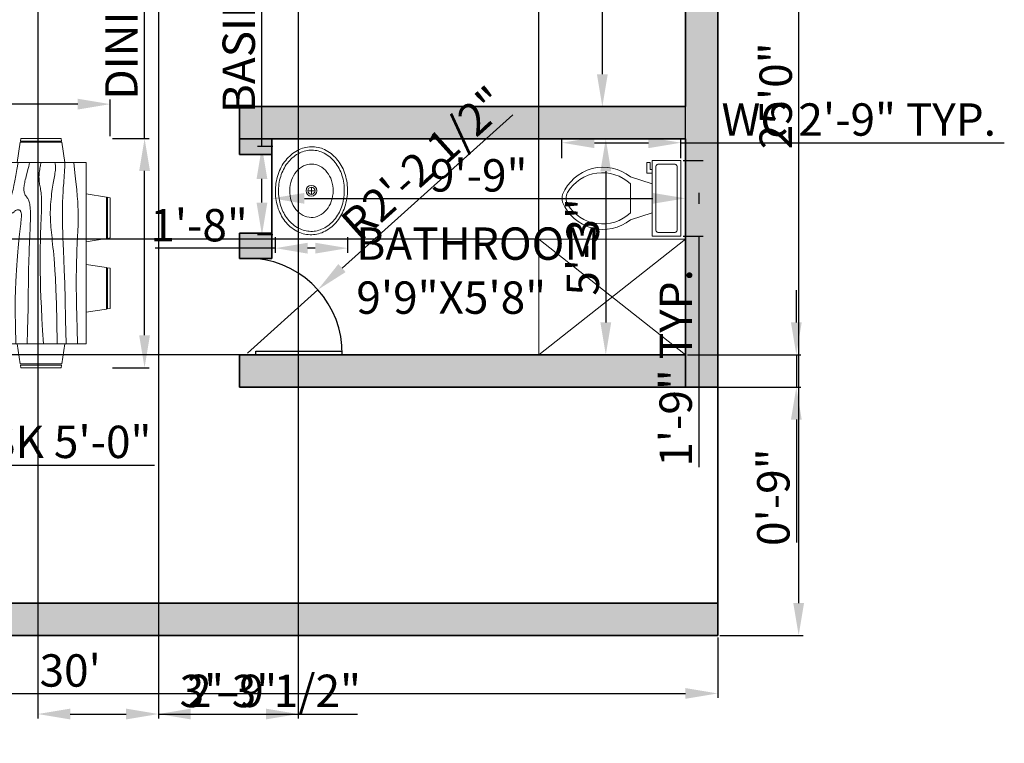
# Model space of a CAD drawing. Units: inches. Extents: x 39700 to 40173, y 40700 to 41139.
# Tile 3 of 4: x 39899 to 40173, y 40718 to 40919. Entities that reach past the tile are written whole.
import ezdxf

# ---------------------------------------------------------------- set-up
doc = ezdxf.new("R2010")
doc.units = ezdxf.units.IN
for name, color, linetype, lineweight in [('A-ANNO-DIMS', 2, 'Continuous', 18), ('A-AREA-IDEN', 7, 'Continuous', 25), ('A-DOOR', 4, 'Continuous', 25), ('A-FLOR-FIXT', 9, 'Continuous', 18), ('A-FURN', 8, 'Continuous', 18), ('A-WALL', 7, 'Continuous', 35)]:
    doc.layers.add(name, color=color, linetype=linetype, lineweight=lineweight)
doc.layers.add('A-WALL-PATT', color=251, linetype='Continuous', lineweight=13, true_color=0x636466)
doc.styles.get("Standard").update_dxf_attribs({"font": 'arial.ttf'})
doc.dimstyles.new('ISO-25', dxfattribs={"dimtxt": 9, "dimasz": 9, "dimexe": 1.25, "dimexo": 0.625, "dimtad": 1, "dimdec": 1, "dimrnd": 9, "dimlunit": 3, "dimtxsty": 'Standard', "dimcen": 2.5, "dimadec": 0, "dimazin": 0, "dimtfac": 1, "dimtdec": 1, "dimtmove": 0, "dimatfit": 3, "dimfxl": 1, "dimarcsym": 0})

# ---------------------------------------------------------------- blocks, each defined once
blk = doc.blocks.new('*D6')
at = {"layer": 'A-ANNO-DIMS', "color": 0, "lineweight": -2, "transparency": 16777216}
for p, q in [((40083.8, 41039.04), (40060.09, 41039.04)), ((40061.34, 41030.04), (40061.34, 40904.04)), ((40083.8, 40895.04), (40060.09, 40895.04))]:
    blk.add_line(p, q, dxfattribs=at)
at = {"layer": 'A-ANNO-DIMS', "color": 0, "transparency": 16777216}
for points in [[(40059.84, 41030.04), (40062.84, 41030.04), (40061.34, 41039.04)], [(40059.84, 40904.04), (40062.84, 40904.04), (40061.34, 40895.04)]]:
    blk.add_solid(points, dxfattribs=at)
at = {"layer": 'Defpoints', "color": 0, "transparency": 16777216}
for p in [(40084.42, 41039.04), (40061.34, 40895.04), (40084.42, 40895.04)]:
    blk.add_point(p, dxfattribs=at)
at = {"layer": 'A-ANNO-DIMS', "color": 0, "transparency": 16777216, "insert": (40056.19, 40967.04), "char_height": 9, "attachment_point": 5, "rotation": 90}
blk.add_mtext("12'", dxfattribs=at)
blk = doc.blocks.new('*D7')
at = {"layer": 'A-ANNO-DIMS', "color": 0, "lineweight": -2, "transparency": 16777216}
for p, q in [((40083.8, 40886.04), (40061.05, 40886.04)), ((40062.3, 40877.04), (40062.3, 40835.04)), ((40083.8, 40826.04), (40061.05, 40826.04))]:
    blk.add_line(p, q, dxfattribs=at)
at = {"layer": 'A-ANNO-DIMS', "color": 0, "transparency": 16777216}
for points in [[(40060.8, 40877.04), (40063.8, 40877.04), (40062.3, 40886.04)], [(40060.8, 40835.04), (40063.8, 40835.04), (40062.3, 40826.04)]]:
    blk.add_solid(points, dxfattribs=at)
at = {"layer": 'Defpoints', "color": 0, "transparency": 16777216}
for p in [(40084.42, 40886.04), (40062.3, 40826.04), (40084.42, 40826.04)]:
    blk.add_point(p, dxfattribs=at)
at = {"layer": 'A-ANNO-DIMS', "color": 0, "transparency": 16777216, "insert": (40057.08, 40856.04), "char_height": 9, "attachment_point": 5, "rotation": 90}
blk.add_mtext('5\'-3"', dxfattribs=at)
blk = doc.blocks.new('*D10')
at = {"layer": 'A-ANNO-DIMS', "color": 0, "lineweight": -2, "transparency": 16777216}
for p, q in [((40094.05, 41048.04), (40117.17, 41048.04)), ((40115.92, 40757.04), (40115.92, 41039.04)), ((40094.05, 40748.04), (40117.17, 40748.04))]:
    blk.add_line(p, q, dxfattribs=at)
at = {"layer": 'A-ANNO-DIMS', "color": 0, "transparency": 16777216}
for points in [[(40114.42, 41039.04), (40117.42, 41039.04), (40115.92, 41048.04)], [(40114.42, 40757.04), (40117.42, 40757.04), (40115.92, 40748.04)]]:
    blk.add_solid(points, dxfattribs=at)
at = {"layer": 'Defpoints', "color": 0, "transparency": 16777216}
for p in [(40093.42, 41048.04), (40115.92, 41048.04), (40093.42, 40748.04)]:
    blk.add_point(p, dxfattribs=at)
at = {"layer": 'A-ANNO-DIMS', "color": 0, "transparency": 16777216, "insert": (40110.7, 40898.04), "char_height": 9, "attachment_point": 5, "rotation": 90}
blk.add_mtext('25\'0"', dxfattribs=at)
blk = doc.blocks.new('Toilet - top')
for p, q in [((9.5, -6), (9.5, -2)), ((-8, -8.5), (-8, -8)), ((-7, -8), (-7, -9.5)), ((-4, -8), (-6, -14)), ((4, -8), (6, -14)), ((-10, -8.5), (-8, -8.5)), ((-10, -9.5), (-10, -8.5)), ((-7, -9.5), (-10, -9.5)), ((4, -14), (-4, -14))]:
    blk.add_line(p, q)
blk.add_lwpolyline([(10.5, -8), (10.5, 0), (-10.5, 0), (-10.5, -8)], close=True)
for points in [[(-9.5, -2), (-9.5, -6)], [(8.5, -1), (-8.5, -1)], [(-8.5, -7), (8.5, -7)]]:
    blk.add_lwpolyline(points)
for centre, radius, start, end in [((-8.62, -1.88), 0.884, 81.8699, 188.1301), ((8.62, -1.88), 0.884, 351.8699, 98.1301), ((-8.62, -6.12), 0.884, 171.8699, 278.1301), ((8.62, -6.12), 0.884, 261.8699, 8.1301), ((3.52, -21.58), 12.17, 141.4691, 247.9714), ((4.2, -21.82), 11.33, 136.3677, 238.9468), ((-3.52, -21.58), 12.17, 292.0284, 38.5307), ((-4.2, -21.82), 11.33, 301.053, 43.6321), ((0, -27.88), 4, 245.7318, 294.2682), ((0, -29), 4, 254.8605, 285.1395)]:
    blk.add_arc(centre, radius, start, end)
blk = doc.blocks.new('*D20')
at = {"layer": 'A-ANNO-DIMS', "color": 0, "lineweight": -2, "transparency": 16777216}
for p, q in [((39969.51, 40881.12), (39969.51, 40868.28)), ((40084.42, 40881.12), (40084.42, 40868.28)), ((39978.51, 40869.53), (40075.42, 40869.53))]:
    blk.add_line(p, q, dxfattribs=at)
at = {"layer": 'A-ANNO-DIMS', "color": 0, "transparency": 16777216}
for points in [[(39978.51, 40871.03), (39978.51, 40868.03), (39969.51, 40869.53)], [(40075.42, 40871.03), (40075.42, 40868.03), (40084.42, 40869.53)]]:
    blk.add_solid(points, dxfattribs=at)
at = {"layer": 'Defpoints', "color": 0, "transparency": 16777216}
for p in [(39969.51, 40881.75), (40084.42, 40881.75), (40084.42, 40869.53)]:
    blk.add_point(p, dxfattribs=at)
at = {"layer": 'A-ANNO-DIMS', "color": 0, "transparency": 16777216, "insert": (40026.97, 40874.75), "char_height": 9, "attachment_point": 5}
blk.add_mtext('9\'-9"', dxfattribs=at)
blk = doc.blocks.new('Dining Set - 36 x 72 in.')
for p, q in [((-22, 27.5), (-22.1562, 26.50042)), ((-22, 27.5), (-6, 27.5)), ((-5.8437, 26.49966), (-6, 27.5)), ((6, 27.5), (5.8438, 26.50042)), ((6, 27.5), (22, 27.5)), ((22.1563, 26.49966), (22, 27.5)), ((-22.2343, 26.00059), (-23.4847, 17.99762)), ((-22.2304, 26), (-5.7608, 26)), ((-5.8416, 26.5), (-22.1534, 26.5)), ((-4.5152, 17.99762), (-5.7655, 25.99926)), ((5.7657, 26.00059), (4.5153, 17.99762)), ((5.7696, 26), (22.2392, 26)), ((22.1584, 26.5), (5.8466, 26.5)), ((23.4848, 17.99762), (22.2345, 25.99926)), ((36, 18), (-36, 18)), ((-36, 18), (-36, -18)), ((36, -18), (36, 18)), ((-45.5, 8), (-44.5004, 8.15617)), ((-45.5, 8), (-45.5, -8)), ((-44.5, -8.15843), (-44.5, 8.15338)), ((-44.0006, 8.23428), (-35.9976, 9.48474)), ((-44, 8.23041), (-44, -8.23915)), ((44.0006, 8.23428), (35.9976, 9.48474)), ((44, 8.23041), (44, -8.23915)), ((44.5, -8.15843), (44.5, 8.15338)), ((45.5, 8), (44.5005, 8.15617)), ((45.5, 8), (45.5, -8)), ((-44.4997, -8.15631), (-45.5, -8)), ((-35.9976, -9.48476), (-43.9993, -8.2345)), ((35.9976, -9.48476), (43.9993, -8.2345)), ((44.4997, -8.15631), (45.5, -8)), ((-36, -18), (36, -18)), ((-22.2343, -26.0006), (-23.4847, -17.99762)), ((-4.5152, -17.99762), (-5.7655, -25.99928)), ((5.7657, -26.0006), (4.5153, -17.99762)), ((23.4848, -17.99762), (22.2345, -25.99928)), ((-22.2304, -26), (-5.7608, -26)), ((-22, -27.5), (-22.1562, -26.50044)), ((-5.8416, -26.5), (-22.1534, -26.5)), ((-5.8437, -26.49967), (-6, -27.5)), ((5.7696, -26), (22.2392, -26)), ((6, -27.5), (5.8438, -26.50044)), ((22.1584, -26.5), (5.8466, -26.5)), ((22.1563, -26.49967), (22, -27.5)), ((-22, -27.5), (-6, -27.5)), ((6, -27.5), (22, -27.5))]:
    blk.add_line(p, q)
for points in [[(-36, 15), (-31.1772, 14.97754), (-26.8079, 14.91406), (-22.8538, 14.81543), (-19.276, 14.6875), (-16.0362, 14.53613), (-13.0957, 14.36718), (-10.4159, 14.18652), (-7.9583, 14), (-5.6904, 13.81315), (-3.6035, 13.63021), (-1.6954, 13.45508), (0.0365, 13.29166), (1.5945, 13.14388), (2.9811, 13.01562), (4.1988, 12.9108), (5.25, 12.83333), (6.1393, 12.78613), (6.8802, 12.76823), (7.4883, 12.77767), (7.9792, 12.8125), (8.3685, 12.87077), (8.6719, 12.95052), (8.9049, 13.0498), (9.0833, 13.16666), (9.2205, 13.29899), (9.3216, 13.44401), (9.3895, 13.59879), (9.4271, 13.76041), (9.4373, 13.92594), (9.4232, 14.09245), (9.3875, 14.257), (9.3333, 14.41666), (9.2638, 14.56917), (9.1836, 14.71484), (9.0975, 14.85465), (9.0104, 14.98958), (8.9272, 15.1206), (8.8529, 15.2487), (8.7922, 15.37483), (8.75, 15.5), (8.7305, 15.62467), (8.7344, 15.74739), (8.7617, 15.86621), (8.8125, 15.97916), (8.8867, 16.08431), (8.9844, 16.17968), (9.1055, 16.26334), (9.25, 16.33333), (9.4189, 16.38802), (9.6172, 16.42708), (9.8506, 16.45052), (10.125, 16.45833), (10.4463, 16.45052), (10.8203, 16.42708), (11.2529, 16.38802), (11.75, 16.33333), (12.3184, 16.26318), (12.9694, 16.17838), (13.7151, 16.07991), (14.5677, 15.96875), (15.5395, 15.84586), (16.6426, 15.71224), (17.8893, 15.56884), (19.2917, 15.41666), (20.859, 15.25667), (22.5879, 15.08984), (24.4721, 14.91715), (26.5052, 14.73958), (28.6809, 14.5581), (30.9929, 14.3737), (33.4347, 14.18733), (36, 14)], [(-36, 10), (-28.9766, 10.14274), (-23.1725, 10.20442), (-18.4241, 10.19775), (-14.5677, 10.13541), (-11.4399, 10.03011), (-8.877, 9.89453), (-6.7154, 9.74137), (-4.7917, 9.58333), (-2.9698, 9.43082), (-1.2246, 9.28515), (0.4415, 9.14534), (2.026, 9.01041), (3.5266, 8.87939), (4.9408, 8.7513), (6.266, 8.62516), (7.5, 8.5), (8.6411, 8.37549), (9.6914, 8.2539), (10.6538, 8.13818), (11.5312, 8.03125), (12.3267, 7.93603), (13.043, 7.85547), (13.6831, 7.79248), (14.25, 7.75), (14.7471, 7.7303), (15.1797, 7.73307), (15.5537, 7.75732), (15.875, 7.80208), (16.1494, 7.86637), (16.3828, 7.94922), (16.5811, 8.04964), (16.75, 8.16666), (16.8944, 8.29915), (17.0143, 8.44531), (17.1089, 8.60319), (17.1771, 8.77083), (17.218, 8.94629), (17.2305, 9.1276), (17.2137, 9.31282), (17.1667, 9.5), (17.0895, 9.6875), (16.987, 9.875), (16.8649, 10.0625), (16.7292, 10.25), (16.5856, 10.4375), (16.4401, 10.625), (16.2985, 10.8125), (16.1667, 11), (16.05, 11.18733), (15.9518, 11.3737), (15.8752, 11.5581), (15.8229, 11.73958), (15.798, 11.91715), (15.8034, 12.08984), (15.842, 12.25667), (15.9167, 12.41666), (16.0295, 12.56836), (16.1784, 12.70833), (16.3605, 12.83268), (16.5729, 12.9375), (16.8127, 13.01888), (17.0768, 13.07291), (17.3625, 13.0957), (17.6667, 13.08333), (17.9894, 13.03312), (18.3418, 12.94726), (18.7382, 12.82918), (19.1927, 12.68229), (19.7195, 12.51001), (20.3327, 12.31575), (21.0465, 12.10294), (21.875, 11.875), (22.8357, 11.63354), (23.959, 11.37304), (25.2786, 11.08618), (26.8282, 10.76562), (28.6414, 10.40405), (30.752, 9.99414), (33.1936, 9.52856), (36, 9)], [(-36, 5.5), (-30.7157, 5.3348), (-26.069, 5.20963), (-21.9946, 5.11767), (-18.4271, 5.05208), (-15.3009, 5.00602), (-12.5508, 4.97265), (-10.1112, 4.94515), (-7.9167, 4.91666), (-5.909, 4.88167), (-4.0586, 4.83984), (-2.3429, 4.79215), (-0.7396, 4.73958), (0.7739, 4.6831), (2.22, 4.6237), (3.6213, 4.56233), (5, 4.5), (6.373, 4.43782), (7.7344, 4.3776), (9.0723, 4.32129), (10.375, 4.27083), (11.6309, 4.22819), (12.8281, 4.19531), (13.9551, 4.17415), (15, 4.16666), (15.954, 4.17448), (16.819, 4.19791), (17.6001, 4.23698), (18.3021, 4.29166), (18.9299, 4.36198), (19.4883, 4.44791), (19.9823, 4.54948), (20.4167, 4.66666), (20.7969, 4.79899), (21.1302, 4.94401), (21.4245, 5.09879), (21.6875, 5.26041), (21.9271, 5.42594), (22.1511, 5.59245), (22.3672, 5.757), (22.5834, 5.91666), (22.8065, 6.06868), (23.0404, 6.21093), (23.2879, 6.34147), (23.5521, 6.45833), (23.8358, 6.55957), (24.142, 6.64323), (24.4735, 6.70735), (24.8334, 6.75), (25.2235, 6.76969), (25.642, 6.76692), (26.0858, 6.74267), (26.5521, 6.69791), (27.0379, 6.63362), (27.5404, 6.55078), (28.0565, 6.45036), (28.5834, 6.33333), (29.1242, 6.19987), (29.7071, 6.04687), (30.3661, 5.87044), (31.1354, 5.66666), (32.0493, 5.43164), (33.142, 5.16146), (34.4475, 4.85221), (36, 4.5)], [(-36, -1), (-30.7915, -0.6591), (-26.0195, -0.38216), (-21.6519, -0.16284), (-17.6563, 0.00521), (-14.0005, 0.12833), (-10.6523, 0.21289), (-7.5796, 0.26522), (-4.75, 0.29166), (-2.134, 0.29793), (0.2878, 0.28711), (2.5317, 0.26163), (4.6146, 0.22396), (6.5529, 0.17651), (8.3633, 0.12174), (10.0623, 0.06209), (11.6667, 0), (13.1899, -0.06201), (14.6341, -0.1211), (15.9982, -0.17432), (17.2813, -0.21875), (18.4823, -0.25147), (19.6003, -0.26953), (20.6343, -0.27002), (21.5834, -0.25), (22.4481, -0.20768), (23.2357, -0.14584), (23.9549, -0.06836), (24.6146, 0.02083), (25.2235, 0.11784), (25.7904, 0.21875), (26.3241, 0.31966), (26.8334, 0.41666), (27.3265, 0.50618), (27.8099, 0.58593), (28.2894, 0.65397), (28.7709, 0.70833), (29.2601, 0.74707), (29.763, 0.76823), (30.2855, 0.76985), (30.8334, 0.75), (31.4088, 0.70784), (31.9994, 0.64713), (32.589, 0.57275), (33.1615, 0.48958), (33.7008, 0.4025), (34.1908, 0.3164), (34.6153, 0.23616), (34.9584, 0.16666), (35.2099, 0.11165), (35.3848, 0.07031), (35.504, 0.04069), (35.5886, 0.02083), (35.6594, 0.00879), (35.7377, 0.0026), (35.8442, 0.00032), (36, 0)], [(-36, -6.5), (-27.1843, -6.31267), (-20.084, -6.1263), (-14.469, -5.9419), (-10.1094, -5.76042), (-6.7752, -5.58285), (-4.2363, -5.41016), (-2.2629, -5.24333), (-0.625, -5.08334), (0.8708, -4.93099), (2.2715, -4.78646), (3.5872, -4.64974), (4.8281, -4.52084), (6.0046, -4.39974), (7.127, -4.28646), (8.2053, -4.18099), (9.25, -4.08334), (10.2705, -3.99382), (11.2734, -3.91407), (12.2647, -3.84603), (13.25, -3.79167), (14.2354, -3.75293), (15.2266, -3.73177), (16.2295, -3.73015), (17.25, -3.75), (18.2912, -3.79248), (19.3451, -3.85547), (20.4009, -3.93604), (21.4479, -4.03125), (22.4754, -4.13819), (23.4727, -4.25391), (24.4289, -4.37549), (25.3334, -4.5), (26.1785, -4.62492), (26.9694, -4.74935), (27.7145, -4.87281), (28.4219, -4.99479), (29.1, -5.11483), (29.7572, -5.23242), (30.4016, -5.34709), (31.0417, -5.45834), (31.6837, -5.56437), (32.3262, -5.65821), (32.9658, -5.73153), (33.599, -5.77604), (34.2224, -5.78345), (34.8327, -5.74545), (35.4264, -5.65373), (36, -5.5)], [(-36, -10), (-26.4022, -9.81299), (-18.4675, -9.62891), (-11.9839, -9.45069), (-6.7396, -9.28125), (-2.5226, -9.12354), (0.8789, -8.98047), (3.6769, -8.85498), (6.0833, -8.75), (8.2767, -8.66765), (10.3021, -8.60677), (12.1712, -8.56543), (13.8958, -8.54167), (15.4876, -8.53353), (16.9583, -8.53907), (18.3197, -8.55632), (19.5834, -8.58334), (20.7616, -8.61841), (21.8685, -8.66081), (22.9188, -8.71004), (23.9271, -8.76563), (24.9081, -8.82707), (25.8763, -8.89388), (26.8465, -8.96558), (27.8334, -9.04167), (28.8474, -9.12118), (29.8828, -9.20117), (30.93, -9.27824), (31.9792, -9.34896), (33.0205, -9.40991), (34.0443, -9.45768), (35.0407, -9.48885), (36, -9.5)], [(-36, -14.5), (-30.0881, -14.33513), (-25.0332, -14.21224), (-20.7312, -14.12647), (-17.0781, -14.07292), (-13.97, -14.04671), (-11.3027, -14.04297), (-8.9724, -14.05681), (-6.875, -14.08334), (-4.9224, -14.11833), (-3.0905, -14.16016), (-1.3709, -14.20785), (0.2448, -14.26042), (1.7647, -14.3169), (3.1973, -14.3763), (4.5507, -14.43767), (5.8333, -14.5), (7.0554, -14.5621), (8.235, -14.62175), (9.3922, -14.67652), (10.5469, -14.72396), (11.7192, -14.76164), (12.929, -14.78711), (14.1965, -14.79794), (15.5417, -14.79167), (16.9933, -14.76424), (18.6152, -14.70508), (20.4804, -14.60197), (22.6615, -14.44271), (25.2312, -14.21509), (28.2624, -13.9069), (31.8277, -13.50594), (36, -13)]]:
    blk.add_lwpolyline(points)
blk = doc.blocks.new('*D21')
at = {"layer": 'A-ANNO-DIMS', "color": 0, "lineweight": -2, "transparency": 16777216}
for p, q in [((39733.42, 40747.42), (39733.42, 40730.66)), ((40093.42, 40747.42), (40093.42, 40730.66)), ((39742.42, 40731.91), (40084.42, 40731.91))]:
    blk.add_line(p, q, dxfattribs=at)
at = {"layer": 'A-ANNO-DIMS', "color": 0, "transparency": 16777216}
for points in [[(39742.42, 40733.41), (39742.42, 40730.41), (39733.42, 40731.91)], [(40084.42, 40733.41), (40084.42, 40730.41), (40093.42, 40731.91)]]:
    blk.add_solid(points, dxfattribs=at)
at = {"layer": 'Defpoints', "color": 0, "transparency": 16777216}
for p in [(39733.42, 40748.04), (40093.42, 40748.04), (40093.42, 40731.91)]:
    blk.add_point(p, dxfattribs=at)
at = {"layer": 'A-ANNO-DIMS', "color": 0, "transparency": 16777216, "insert": (39913.42, 40737.13), "char_height": 9, "attachment_point": 5}
blk.add_mtext("30'", dxfattribs=at)
blk = doc.blocks.new('Sink - Oval top')
for p, q in [((-1, 0), (1, 0)), ((0, 1), (0, -1))]:
    blk.add_line(p, q)
for points in [[(-12.23, 0.39, 0.117634), (-11.46, -3.36, 0.104469), (-8.88, -6.8, 0.090016), (-5.08, -9.07, 0.08192), (-0.32, -10.02, 0.08192), (4.49, -9.38, 0.090016), (8.42, -7.36, 0.104469), (11.22, -4.09, 0.117634), (12.23, -0.39, 0.117634), (11.46, 3.36, 0.104469), (8.88, 6.8, 0.090016), (5.08, 9.07, 0.08192), (0.32, 10.02, 0.08192), (-4.49, 9.38, 0.090016), (-8.42, 7.36, 0.104469), (-11.22, 4.09, 0.117634)], [(-11.29, 0.16, 0.118622), (-10.52, -3.25, 0.104678), (-8.07, -6.36, 0.089562), (-4.54, -8.37, 0.081185), (-0.13, -9.15, 0.081185), (4.3, -8.49, 0.089562), (7.89, -6.58, 0.104678), (10.42, -3.55, 0.118622), (11.29, -0.16, 0.118622), (10.52, 3.25, 0.104678), (8.07, 6.36, 0.089562), (4.54, 8.37, 0.081185), (0.13, 9.15, 0.081185), (-4.3, 8.49, 0.089562), (-7.89, 6.58, 0.104678), (-10.42, 3.55, 0.118622)], [(-7.42, 0.08, 0.118283), (-6.91, -2.17, 0.104607), (-5.29, -4.21, 0.089718), (-2.97, -5.53, 0.081436), (-0.07, -6.04, 0.081436), (2.84, -5.59, 0.089718), (5.2, -4.33, 0.104607), (6.86, -2.32, 0.118283), (7.42, -0.08, 0.118283), (6.91, 2.17, 0.104607), (5.29, 4.21, 0.089718), (2.97, 5.53, 0.081436), (0.07, 6.04, 0.081436), (-2.84, 5.59, 0.089718), (-5.2, 4.33, 0.104607), (-6.86, 2.32, 0.118283)]]:
    blk.add_lwpolyline(points, format="xyb", close=True)
for radius in [1.5, 1]:
    blk.add_circle((0, 0), radius)
blk = doc.blocks.new('*D22')
at = {"layer": 'A-ANNO-DIMS', "color": 0, "lineweight": -2, "transparency": 16777216}
for p, q in [((40050.12, 40880.66), (40050.12, 40886.24)), ((40059.12, 40884.99), (40074.17, 40884.99)), ((40083.17, 40880.66), (40083.17, 40886.24)), ((40083.17, 40884.99), (40173.08, 40884.99))]:
    blk.add_line(p, q, dxfattribs=at)
at = {"layer": 'A-ANNO-DIMS', "color": 0, "transparency": 16777216}
for points in [[(40059.12, 40886.49), (40059.12, 40883.49), (40050.12, 40884.99)], [(40074.17, 40886.49), (40074.17, 40883.49), (40083.17, 40884.99)]]:
    blk.add_solid(points, dxfattribs=at)
at = {"layer": 'Defpoints', "color": 0, "transparency": 16777216}
for p in [(40083.17, 40884.99), (40050.12, 40880.03), (40083.17, 40880.03)]:
    blk.add_point(p, dxfattribs=at)
at = {"layer": 'A-ANNO-DIMS', "color": 0, "transparency": 16777216, "insert": (40132.62, 40890.27), "char_height": 9, "attachment_point": 5}
blk.add_mtext('WC 2\'-9" TYP.', dxfattribs=at)
blk = doc.blocks.new('*D23')
at = {"layer": 'A-ANNO-DIMS', "color": 0, "lineweight": -2, "transparency": 16777216}
for p, q in [((40083.79, 40880.03), (40089.37, 40880.03)), ((40088.12, 40871.03), (40088.12, 40868.03)), ((40083.79, 40859.03), (40089.37, 40859.03)), ((40088.12, 40859.03), (40088.12, 40794.77))]:
    blk.add_line(p, q, dxfattribs=at)
at = {"layer": 'A-ANNO-DIMS', "color": 0, "transparency": 16777216}
for points in [[(40086.62, 40871.03), (40089.62, 40871.03), (40088.12, 40880.03)], [(40086.62, 40868.03), (40089.62, 40868.03), (40088.12, 40859.03)]]:
    blk.add_solid(points, dxfattribs=at)
at = {"layer": 'Defpoints', "color": 0, "transparency": 16777216}
for p in [(40083.17, 40880.03), (40083.17, 40859.03), (40088.12, 40859.03)]:
    blk.add_point(p, dxfattribs=at)
at = {"layer": 'A-ANNO-DIMS', "color": 0, "transparency": 16777216, "insert": (40082.9, 40822.4), "char_height": 9, "attachment_point": 5, "rotation": 90}
blk.add_mtext('1\'-9" TYP.', dxfattribs=at)
blk = doc.blocks.new('*D30')
at = {"layer": 'A-ANNO-DIMS', "color": 0, "lineweight": -2, "transparency": 16777216}
for p, q in [((39934.09, 40886.16), (39934.09, 41016.31)), ((39925.16, 40886.16), (39935.34, 40886.16)), ((39934.09, 40831.46), (39934.09, 40877.16)), ((39925.16, 40822.46), (39935.34, 40822.46))]:
    blk.add_line(p, q, dxfattribs=at)
at = {"layer": 'A-ANNO-DIMS', "color": 0, "transparency": 16777216}
for points in [[(39932.59, 40877.16), (39935.59, 40877.16), (39934.09, 40886.16)], [(39932.59, 40831.46), (39935.59, 40831.46), (39934.09, 40822.46)]]:
    blk.add_solid(points, dxfattribs=at)
at = {"layer": 'Defpoints', "color": 0, "transparency": 16777216}
for p in [(39924.53, 40886.16), (39934.09, 40886.16), (39924.53, 40822.46)]:
    blk.add_point(p, dxfattribs=at)
at = {"layer": 'A-ANNO-DIMS', "color": 0, "transparency": 16777216, "insert": (39928.81, 40955.74), "char_height": 9, "attachment_point": 5, "rotation": 90}
blk.add_mtext('DINING SET 5\'-3 1/2"', dxfattribs=at)
blk = doc.blocks.new('*D31')
at = {"layer": 'A-ANNO-DIMS', "color": 0, "lineweight": -2, "transparency": 16777216}
for p, q in [((39886.03, 40895.72), (39830.89, 40895.72)), ((39886.03, 40886.79), (39886.03, 40896.97)), ((39915.53, 40895.72), (39895.03, 40895.72)), ((39924.53, 40886.79), (39924.53, 40896.97))]:
    blk.add_line(p, q, dxfattribs=at)
at = {"layer": 'A-ANNO-DIMS', "color": 0, "transparency": 16777216}
for points in [[(39895.03, 40897.22), (39895.03, 40894.22), (39886.03, 40895.72)], [(39915.53, 40897.22), (39915.53, 40894.22), (39924.53, 40895.72)]]:
    blk.add_solid(points, dxfattribs=at)
at = {"layer": 'Defpoints', "color": 0, "transparency": 16777216}
for p in [(39886.03, 40895.72), (39886.03, 40886.16), (39924.53, 40886.16)]:
    blk.add_point(p, dxfattribs=at)
at = {"layer": 'A-ANNO-DIMS', "color": 0, "transparency": 16777216, "insert": (39853.96, 40901), "char_height": 9, "attachment_point": 5}
blk.add_mtext('3\'-2 1/2"', dxfattribs=at)
blk = doc.blocks.new('*D34')
at = {"layer": 'A-ANNO-DIMS', "color": 0, "lineweight": -2, "transparency": 16777216}
for p, q in [((39805.37, 40803.76), (39805.37, 40794.14)), ((39865.37, 40803.76), (39865.37, 40794.14)), ((39814.37, 40795.39), (39856.37, 40795.39)), ((39865.37, 40795.39), (39936.83, 40795.39))]:
    blk.add_line(p, q, dxfattribs=at)
at = {"layer": 'A-ANNO-DIMS', "color": 0, "transparency": 16777216}
for points in [[(39814.37, 40796.89), (39814.37, 40793.89), (39805.37, 40795.39)], [(39856.37, 40796.89), (39856.37, 40793.89), (39865.37, 40795.39)]]:
    blk.add_solid(points, dxfattribs=at)
at = {"layer": 'Defpoints', "color": 0, "transparency": 16777216}
for p in [(39805.37, 40804.39), (39865.37, 40804.39), (39865.37, 40795.39)]:
    blk.add_point(p, dxfattribs=at)
at = {"layer": 'A-ANNO-DIMS', "color": 0, "transparency": 16777216, "insert": (39905.6, 40800.67), "char_height": 9, "attachment_point": 5}
blk.add_mtext('DESK 5\'-0"', dxfattribs=at)
blk = doc.blocks.new('*D38')
at = {"layer": 'A-ANNO-DIMS', "color": 0, "lineweight": -2, "transparency": 16777216}
for p, q in [((39966.72, 40883.91), (39966.72, 40979.88)), ((39969.78, 40883.91), (39965.47, 40883.91)), ((39966.72, 40868.36), (39966.72, 40874.91)), ((39969.78, 40859.36), (39965.47, 40859.36))]:
    blk.add_line(p, q, dxfattribs=at)
at = {"layer": 'A-ANNO-DIMS', "color": 0, "transparency": 16777216}
for points in [[(39965.22, 40874.91), (39968.22, 40874.91), (39966.72, 40883.91)], [(39965.22, 40868.36), (39968.22, 40868.36), (39966.72, 40859.36)]]:
    blk.add_solid(points, dxfattribs=at)
at = {"layer": 'Defpoints', "color": 0, "transparency": 16777216}
for p in [(39966.72, 40883.91), (39970.4, 40883.91), (39970.4, 40859.36)]:
    blk.add_point(p, dxfattribs=at)
at = {"layer": 'A-ANNO-DIMS', "color": 0, "transparency": 16777216, "insert": (39961.44, 40936.4), "char_height": 9, "attachment_point": 5, "rotation": 90}
blk.add_mtext('BASIN 2\'-0 1/2"', dxfattribs=at)
blk = doc.blocks.new('*D39')
at = {"layer": 'A-ANNO-DIMS', "color": 0, "lineweight": -2, "transparency": 16777216}
for p, q in [((39970.4, 40858.73), (39970.4, 40854.43)), ((39990.54, 40858.73), (39990.54, 40854.43)), ((39970.4, 40855.68), (39937.08, 40855.68)), ((39981.54, 40855.68), (39979.4, 40855.68))]:
    blk.add_line(p, q, dxfattribs=at)
at = {"layer": 'A-ANNO-DIMS', "color": 0, "transparency": 16777216}
for points in [[(39979.4, 40857.18), (39979.4, 40854.18), (39970.4, 40855.68)], [(39981.54, 40857.18), (39981.54, 40854.18), (39990.54, 40855.68)]]:
    blk.add_solid(points, dxfattribs=at)
at = {"layer": 'Defpoints', "color": 0, "transparency": 16777216}
for p in [(39970.4, 40859.36), (39990.54, 40859.36), (39970.4, 40855.68)]:
    blk.add_point(p, dxfattribs=at)
at = {"layer": 'A-ANNO-DIMS', "color": 0, "transparency": 16777216, "insert": (39949.24, 40860.9), "char_height": 9, "attachment_point": 5}
blk.add_mtext('1\'-8"', dxfattribs=at)
blk = doc.blocks.new('*D46')
at = {"layer": 'A-ANNO-DIMS', "color": 0, "lineweight": -2, "transparency": 16777216}
for p, q in [((40115.27, 40835.04), (40115.27, 40844.04)), ((40085.05, 40826.04), (40116.52, 40826.04)), ((40115.27, 40826.04), (40115.27, 40817.04)), ((40085.05, 40817.04), (40116.52, 40817.04)), ((40115.27, 40808.04), (40115.27, 40773.87))]:
    blk.add_line(p, q, dxfattribs=at)
at = {"layer": 'A-ANNO-DIMS', "color": 0, "transparency": 16777216}
for points in [[(40113.77, 40835.04), (40116.77, 40835.04), (40115.27, 40826.04)], [(40113.77, 40808.04), (40116.77, 40808.04), (40115.27, 40817.04)]]:
    blk.add_solid(points, dxfattribs=at)
at = {"layer": 'Defpoints', "color": 0, "transparency": 16777216}
for p in [(40084.42, 40826.04), (40084.42, 40817.04), (40115.27, 40817.04)]:
    blk.add_point(p, dxfattribs=at)
at = {"layer": 'A-ANNO-DIMS', "color": 0, "transparency": 16777216, "insert": (40110.05, 40786.46), "char_height": 9, "attachment_point": 5, "rotation": 90}
blk.add_mtext('0\'-9"', dxfattribs=at)
blk = doc.blocks.new('*D47')
at = {"layer": 'A-ANNO-DIMS', "color": 0, "lineweight": -2, "transparency": 16777216}
for p, q in [((40043.65, 40858.83), (40043.65, 41071.14)), ((40084.42, 40858.83), (40084.42, 41071.14)), ((40052.65, 41069.89), (40075.42, 41069.89))]:
    blk.add_line(p, q, dxfattribs=at)
at = {"layer": 'A-ANNO-DIMS', "color": 0, "transparency": 16777216}
for points in [[(40052.65, 41071.39), (40052.65, 41068.39), (40043.65, 41069.89)], [(40075.42, 41071.39), (40075.42, 41068.39), (40084.42, 41069.89)]]:
    blk.add_solid(points, dxfattribs=at)
at = {"layer": 'Defpoints', "color": 0, "transparency": 16777216}
for p in [(40084.42, 41069.89), (40043.65, 40858.21), (40084.42, 40858.21)]:
    blk.add_point(p, dxfattribs=at)
at = {"layer": 'A-ANNO-DIMS', "color": 0, "transparency": 16777216, "insert": (40064.03, 41075.12), "char_height": 9, "attachment_point": 5}
blk.add_mtext('3\'-5"', dxfattribs=at)
blk = doc.blocks.new('*D48')
at = {"layer": 'A-ANNO-DIMS', "color": 0, "lineweight": -2, "transparency": 16777216}
for p, q in [((40043.02, 40858.21), (39710.32, 40858.21)), ((39711.57, 40835.04), (39711.57, 40849.21)), ((40043.02, 40826.04), (39710.32, 40826.04))]:
    blk.add_line(p, q, dxfattribs=at)
at = {"layer": 'A-ANNO-DIMS', "color": 0, "transparency": 16777216}
for points in [[(39710.07, 40849.21), (39713.07, 40849.21), (39711.57, 40858.21)], [(39710.07, 40835.04), (39713.07, 40835.04), (39711.57, 40826.04)]]:
    blk.add_solid(points, dxfattribs=at)
at = {"layer": 'Defpoints', "color": 0, "transparency": 16777216}
for p in [(39711.57, 40858.21), (40043.65, 40858.21), (40043.65, 40826.04)]:
    blk.add_point(p, dxfattribs=at)
at = {"layer": 'A-ANNO-DIMS', "color": 0, "transparency": 16777216, "insert": (39706.35, 40842.12), "char_height": 9, "attachment_point": 5, "rotation": 90}
blk.add_mtext('2\'-8"', dxfattribs=at)
blk = doc.blocks.new('*D50')
at = {"layer": 'A-ANNO-DIMS', "color": 0, "lineweight": -2, "transparency": 16777216}
for p, q in [((39904.42, 40952.02), (39904.42, 40724.94)), ((39937.94, 40952.02), (39937.94, 40724.94)), ((39913.42, 40726.19), (39928.94, 40726.19)), ((39937.94, 40726.19), (39993.24, 40726.19))]:
    blk.add_line(p, q, dxfattribs=at)
at = {"layer": 'A-ANNO-DIMS', "color": 0, "transparency": 16777216}
for points in [[(39913.42, 40727.69), (39913.42, 40724.69), (39904.42, 40726.19)], [(39928.94, 40727.69), (39928.94, 40724.69), (39937.94, 40726.19)]]:
    blk.add_solid(points, dxfattribs=at)
at = {"layer": 'Defpoints', "color": 0, "transparency": 16777216}
for p in [(39904.42, 40952.64), (39937.94, 40952.64), (39937.94, 40726.19)]:
    blk.add_point(p, dxfattribs=at)
at = {"layer": 'A-ANNO-DIMS', "color": 0, "transparency": 16777216, "insert": (39970.09, 40731.47), "char_height": 9, "attachment_point": 5}
blk.add_mtext('2\'-9 1/2"', dxfattribs=at)
blk = doc.blocks.new('*D51')
at = {"layer": 'A-ANNO-DIMS', "color": 0, "lineweight": -2, "transparency": 16777216}
for p, q in [((39976.83, 40957.96), (39976.83, 40724.94)), ((39937.94, 40952.02), (39937.94, 40724.94)), ((39946.94, 40726.19), (39967.83, 40726.19))]:
    blk.add_line(p, q, dxfattribs=at)
at = {"layer": 'A-ANNO-DIMS', "color": 0, "transparency": 16777216}
for points in [[(39946.94, 40727.69), (39946.94, 40724.69), (39937.94, 40726.19)], [(39967.83, 40727.69), (39967.83, 40724.69), (39976.83, 40726.19)]]:
    blk.add_solid(points, dxfattribs=at)
at = {"layer": 'Defpoints', "color": 0, "transparency": 16777216}
for p in [(39976.83, 40958.58), (39937.94, 40952.64), (39976.83, 40726.19)]:
    blk.add_point(p, dxfattribs=at)
at = {"layer": 'A-ANNO-DIMS', "color": 0, "transparency": 16777216, "insert": (39957.39, 40731.42), "char_height": 9, "attachment_point": 5}
blk.add_mtext('3\'-3"', dxfattribs=at)
blk = doc.blocks.new('*D55')
at = {"layer": 'A-ANNO-DIMS', "color": 0, "lineweight": -2, "transparency": 16777216}
for p, q in [((40036.42, 40892.74), (39988.98, 40850.15)), ((39962.67, 40826.54), (39982.28, 40844.14))]:
    blk.add_line(p, q, dxfattribs=at)
at = {"layer": 'A-ANNO-DIMS', "color": 0, "transparency": 16777216}
blk.add_solid([(39987.97, 40851.27), (39989.98, 40849.04), (39982.28, 40844.14)], dxfattribs=at)
at = {"layer": 'Defpoints', "color": 0, "transparency": 16777216}
for p in [(39982.28, 40844.14), (39962.67, 40826.54)]:
    blk.add_point(p, dxfattribs=at)
at = {"layer": 'A-ANNO-DIMS', "color": 0, "transparency": 16777216, "insert": (40012.52, 40878.38), "char_height": 9, "attachment_point": 5, "rotation": 41.9102}
blk.add_mtext('R2\'-2 1/2"', dxfattribs=at)

msp = doc.modelspace()

# ---------------------------------------------------------------- hatches: boundary and pattern name
at = {"layer": 'A-WALL-PATT'}
h = msp.add_hatch(color=256, dxfattribs=at)
h.dxf.hatch_style = 1
h.paths.add_polyline_path([(39742.42, 41039.04), (39838.42, 41039.04), (39838.42, 40943.28, -0.039113), (39842.92, 40942.53), (39847.42, 40942.53), (39847.42, 40946.04), (39850.1, 40946.04), (39850.1, 40955.04), (39847.42, 40955.04), (39847.42, 41039.04), (39895.42, 41039.04), (39895.42, 40955.04), (39874.1, 40955.04), (39874.1, 40951.54, -0.010637), (39874.1, 40950.54), (39874.1, 40946.04), (39895.42, 40946.04), (39904.42, 40946.04), (39904.42, 41039.04), (40084.42, 41039.04), (40084.42, 40895.04), (39960.51, 40895.04), (39960.51, 40886.04), (40084.42, 40886.04), (40084.42, 40817.04), (40093.42, 40817.04), (40093.42, 41048.04), (39733.42, 41048.04), (39733.42, 40889.95), (39742.42, 40889.95)])
h.paths.add_polyline_path([(39742.42, 40841.95), (39733.42, 40841.95), (39733.42, 40817.06), (39737.92, 40817.06, -0.015901), (39740.88, 40817.06), (39742.42, 40817.06)], flags=17)
h.paths.add_polyline_path([(40093.42, 40757.04), (39796.66, 40757.04), (39796.66, 40748.04), (40093.42, 40748.04)])
h.paths.add_polyline_path([(39753.27, 40757.04), (39742.42, 40757.04), (39742.42, 40769.06), (39733.42, 40769.06), (39733.42, 40748.04), (39753.27, 40748.04)])
h.paths.add_polyline_path([(40084.42, 40826.04), (39960.51, 40826.04), (39960.51, 40817.04), (40084.42, 40817.04)], flags=17)
h.paths.add_polyline_path([(39969.51, 40859.86), (39960.51, 40859.86), (39960.51, 40852.78), (39969.51, 40852.78)], flags=17)
h.paths.add_polyline_path([(39969.51, 40886.04), (39960.51, 40886.04), (39960.51, 40881.75), (39969.51, 40881.75)], flags=17)
h.paths.add_polyline_path([(39852.31, 40989.98), (39900.82, 40989.98), (39900.82, 41008.52), (39852.31, 41008.52)], flags=25)

# ---------------------------------------------------------------- linework, layer by layer
at = {"layer": 'A-DOOR'}
for p, q in [((39965.01, 40826.04), (39965.01, 40827.04)), ((39965.01, 40827.04), (39989.01, 40827.04))]:
    msp.add_line(p, q, dxfattribs=at)
msp.add_arc((39962.67, 40826.54), 26.34, 358.9124, 84.9094, dxfattribs=at)
at = {"layer": 'A-FLOR-FIXT'}
for p, q in [((40084.42, 40858.21), (40043.65, 40858.21)), ((40043.65, 40858.21), (40043.65, 40826.04)), ((40084.42, 40858.21), (40043.65, 40826.04)), ((40043.65, 40858.21), (40084.42, 40826.04))]:
    msp.add_line(p, q, dxfattribs=at)
at = {"layer": 'A-WALL'}
for p, q in [((40093.42, 40748.04), (40093.42, 41048.04)), ((40084.42, 40895.04), (40084.42, 41039.04)), ((40084.42, 40895.04), (39960.51, 40895.04)), ((39960.51, 40895.04), (39960.51, 40881.75)), ((40084.42, 40886.04), (39960.51, 40886.04)), ((39969.51, 40886.04), (39969.51, 40852.78)), ((40084.42, 40817.04), (40084.42, 40886.04)), ((39969.51, 40881.75), (39960.51, 40881.75)), ((39960.51, 40859.86), (39960.51, 40852.78)), ((39960.51, 40859.86), (39969.51, 40859.86)), ((39969.51, 40852.78), (39960.51, 40852.78)), ((40084.42, 40826.04), (39960.51, 40826.04)), ((39960.51, 40826.04), (39960.51, 40817.04)), ((39969.51, 40826.04), (39960.51, 40826.04)), ((40093.42, 40817.04), (39960.51, 40817.04)), ((39796.66, 40757.04), (40093.42, 40757.04)), ((39796.66, 40748.04), (40093.42, 40748.04))]:
    msp.add_line(p, q, dxfattribs=at)

# ---------------------------------------------------------------- block references
at = {"layer": 'A-FLOR-FIXT'}
for name, p, rotation in [('Sink - Oval top', (39980.47, 40871.64), 90), ('Toilet - top', (40083.17, 40869.53), 270)]:
    msp.add_blockref(name, p, dxfattribs=dict(at, rotation=rotation))
at = {"layer": 'A-FURN', "xscale": 0.7, "yscale": 0.7, "rotation": 90}
msp.add_blockref('Dining Set - 36 x 72 in.', (39905.28, 40854.31), dxfattribs=at)

# ---------------------------------------------------------------- texts
at = {"layer": 'A-AREA-IDEN', "insert": (39992.96, 40861.44), "char_height": 9, "attachment_point": 1}
msp.add_mtext_dynamic_manual_height_columns('BATHROOM\\P9\'9"X5\'8"', width=34.373, gutter_width=12.5, heights=[0], dxfattribs=at)

# ---------------------------------------------------------------- dimensions: what is measured, and where the dimension line sits
at = {"layer": 'A-ANNO-DIMS'}
for base, p1, p2, override, picture, middle in [((40084.42, 41069.89), (40043.65, 40858.21), (40084.42, 40858.21), {"dimdec": 1, "dimlfac": 1, "dimrnd": 0, "dimzin": 1, "dimdsep": 46, "dimlunit": 4, "dimfrac": 2}, '*D47', (40064.03, 41075.12)), ((39976.83, 40726.19), (39937.94, 40952.64), (39976.83, 40958.58), {"dimdec": 1, "dimlfac": 1, "dimrnd": 0, "dimzin": 1, "dimdsep": 46, "dimlunit": 4, "dimfrac": 2}, '*D51', (39957.39, 40731.42)), ((39937.94, 40726.19), (39904.42, 40952.64), (39937.94, 40952.64), {"dimdec": 1, "dimlfac": 1, "dimrnd": 0, "dimzin": 1, "dimdsep": 46, "dimlunit": 4, "dimfrac": 2}, '*D50', (39970.09, 40731.47)), ((40084.42, 40869.53), (39969.51, 40881.75), (40084.42, 40881.75), {"dimclrd": 0, "dimclre": 0, "dimclrt": 0}, '*D20', (40026.97, 40874.75)), ((40093.42, 40731.91), (39733.42, 40748.04), (40093.42, 40748.04), {"dimclrd": 0, "dimclre": 0, "dimclrt": 0}, '*D21', (39913.42, 40737.13))]:
    dim = msp.add_linear_dim(base=base, p1=p1, p2=p2, dimstyle='ISO-25', override=override, dxfattribs=at)
    dim.commit()
    dim.dimension.update_dxf_attribs({"geometry": picture, "text_midpoint": middle})
for base, p1, p2, angle, text, override, picture, middle in [((40115.92, 41048.04), (40093.42, 40748.04), (40093.42, 41048.04), 90, '25\'0"', {"dimclrd": 0, "dimclre": 0, "dimclrt": 0}, '*D10', (40110.7, 40898.04)), ((39934.09, 40886.16), (39924.53, 40822.46), (39924.53, 40886.16), 90, 'DINING SET <>', {"dimdec": 1, "dimlfac": 1, "dimrnd": 0, "dimzin": 1, "dimdsep": 46, "dimlunit": 4, "dimfrac": 2}, '*D30', (39928.81, 40955.74)), ((39966.7205, 40883.9107), (39970.4032, 40859.3598), (39970.4032, 40883.9107), 90, 'BASIN <>', {"dimdec": 1, "dimlfac": 1, "dimrnd": 0, "dimzin": 1, "dimdsep": 46, "dimlunit": 4, "dimfrac": 2}, '*D38', (39961.442, 40936.3962)), ((40088.12, 40859.03), (40083.17, 40880.03), (40083.17, 40859.03), 270, '<> TYP.', {"dimdec": 1, "dimlfac": 1, "dimrnd": 0, "dimzin": 1, "dimdsep": 46, "dimlunit": 4, "dimfrac": 2}, '*D23', (40082.9, 40822.4))]:
    dim = msp.add_linear_dim(base=base, p1=p1, p2=p2, angle=angle, text=text, dimstyle='ISO-25', override=override, dxfattribs=at)
    dim.commit()
    dim.dimension.update_dxf_attribs({"geometry": picture, "text_midpoint": middle})
for base, p1, p2, angle, override, picture, middle in [((40061.34, 40895.04), (40084.42, 41039.04), (40084.42, 40895.04), 90, {"dimclrd": 0, "dimclre": 0, "dimclrt": 0}, '*D6', (40056.19, 40967.04)), ((39886.03, 40895.72), (39924.53, 40886.16), (39886.03, 40886.16), 180, {"dimdec": 1, "dimlfac": 1, "dimrnd": 0, "dimzin": 1, "dimdsep": 46, "dimlunit": 4, "dimfrac": 2}, '*D31', (39853.96, 40901)), ((40062.3, 40826.04), (40084.42, 40886.04), (40084.42, 40826.04), 90, {"dimclrd": 0, "dimclre": 0, "dimclrt": 0}, '*D7', (40057.08, 40856.04)), ((39970.4, 40855.68), (39990.54, 40859.36), (39970.4, 40859.36), 180, {"dimdec": 1, "dimlfac": 1, "dimrnd": 0, "dimzin": 1, "dimdsep": 46, "dimlunit": 4, "dimfrac": 2}, '*D39', (39949.24, 40860.9)), ((39711.57, 40858.21), (40043.65, 40826.04), (40043.65, 40858.21), 90, {"dimdec": 1, "dimlfac": 1, "dimrnd": 0, "dimzin": 1, "dimdsep": 46, "dimlunit": 4, "dimfrac": 2}, '*D48', (39706.35, 40842.12)), ((40115.27, 40817.04), (40084.42, 40826.04), (40084.42, 40817.04), 90, {"dimdec": 1, "dimlfac": 1, "dimrnd": 0, "dimzin": 1, "dimdsep": 46, "dimlunit": 4, "dimfrac": 2}, '*D46', (40110.05, 40786.46))]:
    dim = msp.add_linear_dim(base=base, p1=p1, p2=p2, angle=angle, dimstyle='ISO-25', override=override, dxfattribs=at)
    dim.commit()
    dim.dimension.update_dxf_attribs({"geometry": picture, "text_midpoint": middle})
for base, p1, p2, text, picture, middle in [((40083.1656, 40884.9909), (40050.1194, 40880.034), (40083.1656, 40880.034), 'WC <> TYP.', '*D22', (40132.6246, 40890.2694)), ((39865.37, 40795.39), (39805.37, 40804.39), (39865.37, 40804.39), 'DESK <>', '*D34', (39905.6, 40800.67))]:
    dim = msp.add_linear_dim(base=base, p1=p1, p2=p2, text=text, dimstyle='ISO-25', override={"dimdec": 1, "dimlfac": 1, "dimrnd": 0, "dimzin": 1, "dimdsep": 46, "dimlunit": 4, "dimfrac": 2}, dxfattribs=at)
    dim.commit()
    dim.dimension.update_dxf_attribs({"geometry": picture, "text_midpoint": middle})
dim = msp.add_radius_dim(center=(39962.67, 40826.54), mpoint=(39982.28, 40844.14), dimstyle='ISO-25', override={"dimdec": 1, "dimlfac": 1, "dimrnd": 0, "dimzin": 1, "dimdsep": 46, "dimlunit": 4, "dimfrac": 2}, dxfattribs=at)
dim.commit()
dim.dimension.update_dxf_attribs({"geometry": '*D55', "text_midpoint": (40012.52, 40878.38)})

doc.saveas('drawing.dxf')
